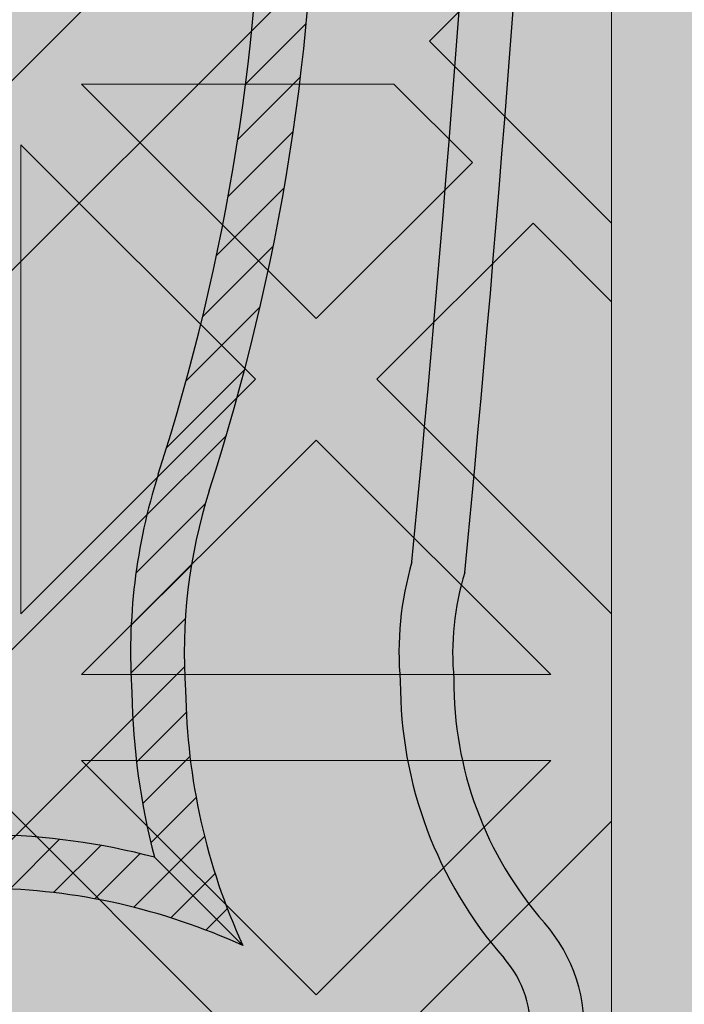
# Model space of a CAD drawing. Units: inches. Extents: x 844 to 2234, y 346 to 1084.
# Tile 10 of 93: x 1125.562 to 1127.536, y 688.258 to 691.183. Entities that reach past the tile are written whole.
import ezdxf

# ---------------------------------------------------------------- set-up
doc = ezdxf.new("R2010")
doc.units = ezdxf.units.IN
doc.header["$MEASUREMENT"] = 0
for name, color, linetype, lineweight in [('A-ANNO-DIMS', 2, 'Continuous', 18), ('furniture', 8, 'Continuous', 18), ('RA-AP-01$0$INT', 35, 'Continuous', 5)]:
    doc.layers.add(name, color=color, linetype=linetype, lineweight=lineweight)
doc.layers.add('RA-AP-01$0$FURN', color=3, linetype='Continuous')
doc.layers.add('RA-AP-01$0$WOOD', color=64, linetype='Continuous')
doc.styles.get("Standard").update_dxf_attribs({"font": 'arial.ttf'})
doc.dimstyles.get("Standard").update_dxf_attribs({"dimtxt": 6, "dimasz": 3, "dimexe": 0.18, "dimexo": 0.0625, "dimgap": 0.09, "dimtad": 0, "dimtih": 1, "dimtoh": 1, "dimdec": 1, "dimzin": 0, "dimdsep": 46, "dimlunit": 3, "dimtxsty": 'Standard', "dimblk": 'ARCHTICK', "dimcen": 0.09, "dimadec": 0, "dimazin": 0, "dimtfac": 1, "dimtdec": 1, "dimtofl": 0, "dimtmove": 0, "dimatfit": 3, "dimfxl": 1, "dimtolj": 1, "dimtzin": 0, "dimarcsym": 0})

# ---------------------------------------------------------------- blocks, each defined once
blk = doc.blocks.new('A$C18D01794')
at = {"layer": 'RA-AP-01$0$INT'}
blk.add_hatch(color=256, dxfattribs=at).paths.add_polyline_path([(4.505206456958071, -6.306712009588038), (5.305206456958072, -6.306712009588038), (5.305206456958072, -7.106712009588038), (5.255206456951893, -7.10671200958804), (5.25520645694868, -6.356712009605972), (4.555206456959269, -6.356712009587461), (4.555206456956052, -7.106712009588038), (4.505206456958073, -7.106712009588038)])
h = blk.add_hatch(color=256, dxfattribs=at)
h.paths.add_polyline_path([(4.585917135068449, -6.356712009588271), (4.555206456959269, -6.35671200958746), (4.555206456959137, -6.387422687716308), (4.874495778835233, -6.706712009592356), (4.90520645695423, -6.676001331474049)])
h.paths.add_polyline_path([(5.255206456948813, -6.387422687716306), (5.255206456948682, -6.356712009605972), (5.224495778822613, -6.356712009605161), (4.905206456953498, -6.676001331474273), (4.935917135072151, -6.706712009592924)])
h.paths.add_polyline_path([(4.935917135072559, -6.706712009592068), (4.905206456953564, -6.737422687710376), (5.255206456951813, -7.087422687708613), (5.255206456951549, -7.026001331471008)])
h.paths.add_polyline_path([(4.555206456956399, -7.026001331471013), (4.555206456956134, -7.087422687708616), (4.905206456953821, -6.737422687710943), (4.874495778835166, -6.70671200959229)])
h = blk.add_hatch(color=256, dxfattribs=at)
h.paths.add_polyline_path([(4.585917135068448, -6.356712009588273), (4.614201406330596, -6.356712009589021), (4.668846067270487, -6.411356670531338), (4.723490728212344, -6.356712009591912), (4.771774999457151, -6.35671200959319), (4.826419660396886, -6.411356670535356), (4.862780050090322, -6.374996280843536), (4.844495778842715, -6.356712009595112), (4.862780050090411, -6.356712009595595), (4.905206456960182, -6.399138416468211), (4.947632863832445, -6.356712009597838), (4.965917135079675, -6.356712009598322), (4.947632863831759, -6.374996280845421), (4.983993253523576, -6.411356670538857), (5.038637914464627, -6.356712009600247), (5.08692218571208, -6.356712009601523), (5.141566846649976, -6.411356670541852), (5.196211507589851, -6.356712009604411), (5.224495778822615, -6.356712009605161), (4.905206456953975, -6.676001331473793)])
h.paths.add_polyline_path([(4.895206456956031, -6.637717060225675), (4.895206456958921, -6.528427738347902), (4.840561796018589, -6.583072399285802)], flags=16)
h.paths.add_polyline_path([(4.915206456955638, -6.637717060226121), (4.969851117895509, -6.583072399288678), (4.915206456957609, -6.528427738348344)], flags=16)
h.paths.add_polyline_path([(4.826419660395175, -6.568930263661755), (4.881064321335613, -6.514285602723745), (4.771774999456703, -6.514285602720857)], flags=16)
h.paths.add_polyline_path([(4.983993253519558, -6.568930263665262), (5.038637914460456, -6.514285602726792), (4.929348592581548, -6.514285602724816)], flags=16)
h.paths.add_polyline_path([(4.881064321336025, -6.494285602723742), (4.826419660397532, -6.439640941782821), (4.771774999457062, -6.494285602720859)], flags=16)
h.paths.add_polyline_path([(4.929348592582019, -6.494285602724817), (5.038637914460982, -6.494285602726792), (4.983993253522945, -6.439640941786327)], flags=16)
h.paths.add_polyline_path([(4.895206456960191, -6.480143467100443), (4.895206456962115, -6.407422687715913), (4.876922185715016, -6.389138416467584), (4.840561796021581, -6.425498806159401)], flags=16)
h.paths.add_polyline_path([(4.915206456958487, -6.480143467100889), (4.969851117899527, -6.425498806162279), (4.933490728206909, -6.389138416468043), (4.9152064569598, -6.40742268771434)], flags=16)
h.paths.add_polyline_path([(4.757632863832376, -6.480143467096812), (4.812277524772842, -6.425498806158772), (4.757632863834348, -6.370854145217844)], flags=16)
h.paths.add_polyline_path([(4.737632863832376, -6.480143467096286), (4.737632863834348, -6.370854145217375), (4.682988202893906, -6.425498806155385)], flags=16)
h.paths.add_polyline_path([(5.05278005008503, -6.480143467103376), (5.052780050087917, -6.370854145224413), (4.998135389146995, -6.425498806162908)], flags=16)
h.paths.add_polyline_path([(5.072780050085024, -6.480143467103744), (5.127424711025931, -6.42549880616527), (5.072780050087916, -6.370854145224832)], flags=16)
h.paths.add_polyline_path([(4.935917135072783, -6.706712009592292), (5.255206456948811, -6.387422687716309), (5.255206456948932, -6.415706958964177), (5.200561796010279, -6.470351619902839), (5.255206456949403, -6.524996280841948), (5.25520645694961, -6.5732805520894), (5.200561796009787, -6.627925213029239), (5.236922185702417, -6.664285602721864), (5.255206456949919, -6.646001331474357), (5.255206456949998, -6.664285602721898), (5.212780050078687, -6.706712009592262), (5.25520645695036, -6.749138416463932), (5.255206456950438, -6.767422687711313), (5.236922185702424, -6.749138416463297), (5.200561796009796, -6.785498806155928), (5.255206456950753, -6.840143467096874), (5.25520645695096, -6.888427738341682), (5.200561796010322, -6.943072399282328), (5.255206456951428, -6.997717060223427), (5.255206456951547, -7.026001331471006)])
h.paths.add_polyline_path([(5.042988202883395, -6.785498806155427), (5.097632863823085, -6.840143467095101), (5.097632863822622, -6.730854145216193)], flags=16)
h.paths.add_polyline_path([(5.028846067259663, -6.771356670531693), (5.083490728198774, -6.716712009592573), (4.974201406321001, -6.716712009593042)], flags=16)
h.paths.add_polyline_path([(5.117632863823087, -6.840143467095186), (5.172277524762331, -6.785498806155926), (5.11763286382262, -6.730854145216225)], flags=16)
h.paths.add_polyline_path([(5.08349072819877, -6.696712009593886), (5.028846067259652, -6.642067348654775), (4.974201406320998, -6.696712009593438)], flags=16)
h.paths.add_polyline_path([(5.131774999446817, -6.854285602718917), (5.186419660386065, -6.799640941779662), (5.241064321325782, -6.854285602719365)], flags=17)
h.paths.add_polyline_path([(5.131774999446228, -6.716712009592374), (5.186419660386065, -6.771356670532194), (5.222780050079488, -6.734996280838764), (5.204495778832781, -6.716712009592063)], flags=16)
h.paths.add_polyline_path([(5.097632863822613, -6.682569873970264), (5.097632863823061, -6.573280552091354), (5.042988202883383, -6.627925213031044)], flags=16)
h.paths.add_polyline_path([(5.131774999446899, -6.874285602718915), (5.241064321325809, -6.874285602719364), (5.186419660386591, -6.928930263658598)], flags=17)
h.paths.add_polyline_path([(5.131774999446226, -6.696712009594078), (5.204495778830767, -6.696712009594374), (5.22278005007868, -6.67842773834687), (5.186419660386049, -6.642067348654249)], flags=16)
h.paths.add_polyline_path([(5.11763286382262, -6.682569873970225), (5.17227752476232, -6.627925213030515), (5.117632863823064, -6.573280552091267)], flags=16)
h.paths.add_polyline_path([(5.186419660386069, -6.613783077405491), (5.241064321325754, -6.559138416465795), (5.131774999446791, -6.559138416466263)], flags=16)
h.paths.add_polyline_path([(5.131774999446872, -6.539138416466263), (5.24106432132578, -6.539138416465794), (5.186419660386554, -6.484493755526573)], flags=16)
h.paths.add_polyline_path([(5.255206456951811, -7.08742268770861), (5.255206456951895, -7.106712009588038), (4.555206456956052, -7.106712009588038), (4.555206456956136, -7.087422687708617), (4.905206456953973, -6.737422687710788)])
h.paths.add_polyline_path([(4.983993253513404, -6.8444937555241), (4.92934859257295, -6.899138416462108), (5.03863791445186, -6.899138416465014)], flags=16)
h.paths.add_polyline_path([(4.969851117889988, -6.83035161990006), (4.915206456952556, -6.775706958960171), (4.915206456949648, -6.884996280837944)], flags=16)
h.paths.add_polyline_path([(4.929348592572535, -6.919138416462105), (4.983993253511019, -6.973783077403037), (5.038637914451496, -6.919138416465012)], flags=16)
h.paths.add_polyline_path([(5.052780050074912, -6.93328055208906), (4.998135389134438, -6.987925213027088), (5.052780050072919, -7.042569873968025)], flags=16)
h.paths.add_polyline_path([(5.07278005007491, -6.933280552089588), (5.072780050072918, -7.042569873968497), (5.127424711013374, -6.987925213030498)], flags=16)
h.paths.add_polyline_path([(4.89520645695295, -6.775706958959721), (4.840561796013067, -6.830351619897157), (4.895206456950961, -6.884996280837494)], flags=16)
h.paths.add_polyline_path([(4.915206456948365, -6.933280552085403), (4.915206456946434, -7.006001331471951), (4.933490728192729, -7.024285602719066), (4.969851117886972, -6.987925213026453)], flags=16)
h.paths.add_polyline_path([(4.881064321327021, -6.899138416461022), (4.82641966038902, -6.84449375552057), (4.771774999448108, -6.899138416459029)], flags=16)
h.paths.add_polyline_path([(4.895206456950073, -6.933280552084951), (4.840561796009022, -6.987925213023558), (4.876922185700835, -7.024285602716997), (4.895206456948749, -7.006001331469487)], flags=16)
h.paths.add_polyline_path([(4.983993253510392, -7.0020673486505), (4.947632863816944, -7.038427738342319), (4.965917135064043, -7.05671200959023), (5.038637914448995, -7.056712009591555)], flags=16)
h.paths.add_polyline_path([(4.881064321326543, -6.91913841646102), (4.771774999447578, -6.919138416459031), (4.826419660385607, -6.973783077399508)], flags=16)
h.paths.add_polyline_path([(4.905206456946447, -7.014285602717636), (4.862780050074785, -7.056712009588352), (4.947632863816685, -7.056712009589775)], flags=16)
h.paths.add_polyline_path([(5.14156684663679, -7.002067348654549), (5.086922185696452, -7.056712009592438), (5.196211507574223, -7.056712009594425)], flags=16)
h.paths.add_polyline_path([(4.8264196603837, -7.002067348646972), (4.771774999442643, -7.056712009585575), (4.8444957788276, -7.056712009587508), (4.862780050075511, -7.038427738340416)], flags=16)
h.paths.add_polyline_path([(4.812277524760289, -6.98792521302292), (4.757632863822258, -6.933280552082447), (4.757632863819352, -7.042569873961408)], flags=16)
h.paths.add_polyline_path([(4.73763286382226, -6.933280552082079), (4.682988202881349, -6.987925213020536), (4.737632863819352, -7.04256987396099)], flags=16)
h.paths.add_polyline_path([(4.723490728195188, -7.056712009584289), (4.668846067257299, -7.002067348643949), (4.614201406317417, -7.056712009581383)], flags=16)
h.paths.add_polyline_path([(4.597632863829262, -6.706712009592262), (4.555206456957951, -6.664285602721896), (4.555206456958029, -6.646001331474357), (4.573490728205535, -6.664285602721864), (4.609851117898167, -6.627925213029238), (4.555206456958338, -6.573280552089402), (4.555206456958546, -6.524996280841952), (4.60985111789767, -6.470351619902839), (4.555206456959015, -6.415706958964177), (4.555206456959138, -6.387422687716309), (4.874495778835167, -6.70671200959229), (4.5552064569564, -7.026001331471015), (4.555206456956523, -6.997717060223433), (4.609851117897629, -6.94307239928233), (4.555206456956988, -6.888427738341681), (4.555206456957198, -6.840143467096881), (4.609851117898153, -6.78549880615593), (4.573490728205528, -6.749138416463297), (4.555206456957507, -6.76742268771132), (4.555206456957585, -6.749138416463933)])
h.paths.add_polyline_path([(4.712780050085332, -6.730854145216195), (4.712780050084863, -6.840143467095105), (4.767424711024555, -6.785498806155427)], flags=16)
h.paths.add_polyline_path([(4.726922185709173, -6.716712009592573), (4.781566846648288, -6.771356670531693), (4.836211507586949, -6.716712009593043)], flags=16)
h.paths.add_polyline_path([(4.692780050085327, -6.730854145216225), (4.638135389145619, -6.785498806155928), (4.692780050084865, -6.840143467095185)], flags=16)
h.paths.add_polyline_path([(4.726922185709182, -6.696712009593886), (4.836211507586949, -6.696712009593436), (4.7815668466483, -6.642067348654773)], flags=16)
h.paths.add_polyline_path([(4.678637914461726, -6.71671200959237), (4.605917135075169, -6.716712009592063), (4.587632863828464, -6.734996280838766), (4.623993253521887, -6.771356670532195)], flags=16)
h.paths.add_polyline_path([(4.712780050085336, -6.68256987397026), (4.767424711024568, -6.627925213031042), (4.71278005008489, -6.573280552091352)], flags=16)
h.paths.add_polyline_path([(4.678637914461726, -6.696712009594076), (4.623993253521899, -6.642067348654247), (4.587632863829271, -6.67842773834687), (4.605917135077185, -6.696712009594376)], flags=16)
h.paths.add_polyline_path([(4.692780050085336, -6.682569873970228), (4.692780050084889, -6.573280552091267), (4.638135389145632, -6.627925213030515)], flags=16)
h.paths.add_polyline_path([(4.623993253521885, -6.799640941779662), (4.678637914461131, -6.854285602718915), (4.56934859258217, -6.854285602719365)], flags=17)
h.paths.add_polyline_path([(4.623993253521901, -6.613783077405509), (4.678637914461158, -6.559138416466263), (4.569348592582195, -6.559138416465795)], flags=16)
h.paths.add_polyline_path([(4.678637914461051, -6.874285602718915), (4.623993253521361, -6.928930263658598), (4.569348592582143, -6.874285602719364)], flags=17)
h.paths.add_polyline_path([(4.678637914461076, -6.539138416466263), (4.623993253521399, -6.484493755526573), (4.569348592582167, -6.539138416465796)], flags=16)
h = blk.add_hatch(color=256, dxfattribs=at)
h.paths.add_polyline_path([(5.028846067259997, -6.642067348655121), (4.974201406321342, -6.696712009593783), (5.083490728199115, -6.69671200959423)])
h.paths.add_polyline_path([(4.974201406321344, -6.716712009593388), (5.028846067260004, -6.771356670532039), (5.083490728199117, -6.716712009592919)])
h.paths.add_polyline_path([(5.042988202883738, -6.785498806155768), (5.097632863823428, -6.840143467095449), (5.097632863822963, -6.73085414521654)])
h.paths.add_polyline_path([(5.117632863822961, -6.730854145216568), (5.117632863823428, -6.840143467095531), (5.172277524762674, -6.785498806156272)])
h.paths.add_polyline_path([(5.131774999446572, -6.716712009592718), (5.186419660386406, -6.77135667053254), (5.222780050079831, -6.734996280839116), (5.204495778833122, -6.716712009592409)])
h.paths.add_polyline_path([(5.236922185702764, -6.749138416463644), (5.200561796010139, -6.785498806156274), (5.255206456949971, -6.840143467096101), (5.255206456950271, -6.76742268771115)])
h.paths.add_polyline_path([(5.186419660386412, -6.799640941780006), (5.131774999447164, -6.854285602719262), (5.241064321326123, -6.854285602719711)])
h.paths.add_polyline_path([(5.131774999447238, -6.874285602719261), (5.186419660386934, -6.928930263658944), (5.241064321326153, -6.874285602719709)])
h.paths.add_polyline_path([(5.200561796010663, -6.943072399282675), (5.255206456949324, -6.997717060221329), (5.255206456949777, -6.888427738343558)])
h.paths.add_polyline_path([(5.21278005007903, -6.706712009592607), (5.255206456950223, -6.749138416463798), (5.255206456950696, -6.664285602721891)])
h.paths.add_polyline_path([(5.13177499944657, -6.696712009594424), (5.204495778831106, -6.696712009594723), (5.222780050079024, -6.678427738347219), (5.186419660386397, -6.642067348654592)])
h.paths.add_polyline_path([(5.117632863823405, -6.573280552091611), (5.117632863822955, -6.682569873970578), (5.172277524762665, -6.627925213030859)])
h.paths.add_polyline_path([(5.042988202883727, -6.627925213031387), (5.097632863822957, -6.682569873970603), (5.097632863823407, -6.573280552091697)])
h.paths.add_polyline_path([(5.131774999447135, -6.559138416466609), (5.186419660386394, -6.613783077405857), (5.241064321326097, -6.559138416466144)])
h.paths.add_polyline_path([(5.200561796010128, -6.627925213029584), (5.236922185702758, -6.664285602722211), (5.255206456950264, -6.646001331474705), (5.255206456949948, -6.573280552089752)])
h.paths.add_polyline_path([(5.186419660386895, -6.484493755526919), (5.131774999447213, -6.539138416466609), (5.241064321326127, -6.539138416466142)])
h.paths.add_polyline_path([(5.200561796010624, -6.470351619903183), (5.255206456949745, -6.524996280842298), (5.255206456949276, -6.415706958964523)])
for p, q in [((5.255206456951895, -7.106712009588038), (5.255206456948681, -6.356712009605972)), ((4.935917135072783, -6.706712009592292), (5.255206456948813, -6.387422687716307)), ((5.255206456949399, -6.524996280841946), (5.200561796010281, -6.470351619902839)), ((5.18641966038655, -6.484493755526575), (5.131774999446872, -6.539138416466263)), ((5.241064321325782, -6.539138416465796), (5.186419660386552, -6.484493755526573)), ((5.131774999446872, -6.539138416466263), (5.241064321325782, -6.539138416465796)), ((5.131774999446792, -6.559138416466263), (5.241064321325755, -6.559138416465795)), ((5.131774999446792, -6.559138416466263), (5.186419660386049, -6.613783077405509)), ((5.241064321325755, -6.559138416465795), (5.186419660386049, -6.613783077405509)), ((5.117632863823062, -6.573280552091267), (5.172277524762319, -6.627925213030515)), ((5.117632863823062, -6.573280552091267), (5.117632863822614, -6.68256987397023)), ((5.255206456949605, -6.573280552089405), (5.200561796009783, -6.627925213029239)), ((5.255206456949918, -6.646001331474357), (5.255206456949605, -6.573280552089405)), ((5.117632863822614, -6.68256987397023), (5.172277524762319, -6.627925213030515)), ((5.200561796009783, -6.627925213029238), (5.236922185702415, -6.664285602721863)), ((5.131774999446228, -6.696712009594078), (5.186419660386053, -6.642067348654247)), ((5.186419660386051, -6.642067348654247), (5.222780050078681, -6.67842773834687)), ((5.255206456949919, -6.646001331474357), (5.236922185702415, -6.664285602721864)), ((5.212780050078687, -6.706712009592262), (5.255206456950353, -6.664285602721543)), ((5.25520645694988, -6.74913841646345), (5.255206456950353, -6.664285602721543)), ((5.204495778833082, -6.69671200959206), (5.222780050078681, -6.67842773834687)), ((5.204495778831179, -6.696712009594376), (5.131774999446228, -6.696712009594078)), ((5.212780050078687, -6.706712009592262), (5.25520645694988, -6.74913841646345))]:
    blk.add_line(p, q, dxfattribs=at)
blk = doc.blocks.new('A$C32926AE1')
at = {"layer": 'RA-AP-01$0$WOOD'}
h = blk.add_hatch(color=256, dxfattribs=at)
h.dxf.hatch_style = 1
h.paths.add_polyline_path([(5.157430609644524, 4.573483066760929, -0.1009492694046607), (5.155401577623758, 4.593365984175333, -0.1842662638101597), (5.172249623284174, 4.638795604568598, 0.2056608120311276), (5.179560981299304, 4.661316324430096, 0.3614336704623542), (5.134352340494423, 4.706524965234944, 0.2056608120311297), (5.111831620632933, 4.699213607219793, -0.1842662638101113), (5.066402000239693, 4.682365561559342, -0.1055311479399994), (5.045656153913092, 4.68467289944697, 0.1567636581983829), (4.763886414745334, 4.684672899446966, -0.1055311479399895), (4.743140568418733, 4.68236556155934, -0.1842662638100833), (4.6977109480255, 4.69921360721979, 0.2056608120302612), (4.675190228164109, 4.706524965234949, 0.3614336704708441), (4.629981587358889, 4.66131632442871, 0.2056608120245944), (4.637292945374126, 4.638795604567974, -0.1842662638101024), (4.654140991034615, 4.59336598417475, -0.1009492694055169), (4.652111959013835, 4.573483066760181, 0.021410119221476), (4.629748025606143, 4.156712009541676, 0.0214101192214795), (4.652111959013809, 3.739940952323101, -0.1009492694059586), (4.654140991034615, 3.720058034908448, -0.1842662638100975), (4.637292945374126, 3.674628414515226, 0.2056608120245705), (4.629981587358889, 3.652107694654492, 0.3614336704708879), (4.675190228164113, 3.606899053848249, 0.2056608120302384), (4.697710948025501, 3.614210411863408, -0.1842662638100995), (4.743140568418738, 3.63105845752386, -0.1055311479402541), (4.763886414745388, 3.628751119636215, 0.1567636581983776), (5.045656153913137, 3.628751119636244, -0.1055311479397538), (5.066402000239692, 3.631058457523857, -0.1842662638101067), (5.111831620632931, 3.614210411863407, 0.2056608120310924), (5.134352340494417, 3.606899053848256, 0.3614336704624001), (5.179560981299307, 3.652107694653103, 0.2056608120311314), (5.172249623284175, 3.6746284145146, -0.1842662638101402), (5.155401577623758, 3.72005803490786, -0.1009492694051366), (5.15743060964455, 3.739940952322354, 0.0214101192215073), (5.179794543052287, 4.156712009541468, 0.0214101192215252)])
h.paths.add_polyline_path([(4.639748609479751, 4.156712009541513, 0.0213537860821624), (4.661970494867118, 3.741887061152232, -0.094075836301374), (4.664143710413708, 3.7196126951003, -0.1824818158568985), (4.644813765429836, 3.668037719127816, 0.2056608120245319), (4.639939526753007, 3.653023905887301, 0.3614336704710246), (4.676106439397173, 3.616856993242342, 0.2056608120302234), (4.691120252638095, 3.621731231919122, -0.1824818158602558), (4.742695228611606, 3.641061176902986, -0.1029891339458722), (4.766991894714349, 3.638256818950944, 0.156709409989566), (5.042550673941472, 3.638256818950105, -0.102989133958497), (5.066847340047078, 3.641061176902949, -0.1824818158594995), (5.118422316020358, 3.621731231919103, 0.2056608120311416), (5.133436129261316, 3.616856993242346, 0.3614336704621468), (5.169603041905217, 3.653023905886178, 0.2056608120310986), (5.164728803228477, 3.668037719127177, -0.1824818158565612), (5.145398858244737, 3.719612695099578, -0.0940758363009313), (5.147572073791232, 3.741887061151398, 0.0213537860822023), (5.169793959178681, 4.156712009541451, 0.0213537860822226), (5.147572073791203, 4.571536957931898, -0.0940758363005034), (5.145398858244737, 4.59381132398362, -0.1824818158565587), (5.164728803228476, 4.645386299956021, 0.2056608120311045), (5.169603041905216, 4.66040011319702, 0.3614336704621845), (5.133436129261313, 4.696567025840856, 0.2056608120310773), (5.118422316020359, 4.691692787164098, -0.182481815859508), (5.066847340047078, 4.67236284218025, -0.1029891339584606), (5.04255067394148, 4.675167200133092, 0.156709409989566), (4.766991894714357, 4.675167200132257, -0.1029891339458842), (4.742695228611611, 4.672362842180213, -0.1824818158602725), (4.691120252638095, 4.691692787164077, 0.2056608120302152), (4.676106439397174, 4.696567025840858, 0.3614336704710363), (4.639939526753005, 4.660400113195899, 0.2056608120245495), (4.644813765429837, 4.645386299955384, -0.1824818158568934), (4.664143710413708, 4.593811323982902, -0.0940758363009187), (4.661970494867149, 4.571536957931074, 0.021353786082177)], flags=16)
h.paths.add_polyline_path([(5.129794543052235, 4.432167055276933, -0.0141661062790638), (5.130152669293814, 4.156927903047693, -0.0141661062790647), (5.129794543052234, 3.881688750818433, -0.0785247771143638), (5.10979738006795, 3.755143611847103, 0.0945969212073497), (5.105408519571111, 3.717898134952927, 0.1043170707844957), (5.116074640131521, 3.670385395016088, 0.1043170707864965), (5.068561900193738, 3.681051515576561, 0.09459692119553), (5.031316423304057, 3.676662655080835, -0.1580239521427272), (4.778226145355827, 3.676662655080367, 0.0945969211986668), (4.740980668464973, 3.681051515576592, 0.1043170707882822), (4.693467928526415, 3.670385395015844, 0.1043170707867916), (4.704134049087309, 3.717898134953662, 0.0945969211972894), (4.69974518859162, 3.755143611844042, -0.0785247771163196), (4.679748025606343, 3.881688750818406, -0.0141661062790663), (4.679389899364763, 4.156927903047693, -0.0141661062790672), (4.679748025606343, 4.432167055276998, -0.0785247771163064), (4.699745188591625, 4.55871219425134, 0.094596921197333), (4.704134049087308, 4.595957671141738, 0.1043170707867205), (4.693467928526416, 4.643470411079523, 0.1043170707882628), (4.740980668464965, 4.632804290518776, 0.0945969211988114), (4.778226145355874, 4.637193151015016, -0.158023952142669), (5.031316423304015, 4.637193151014546, 0.0945969211956361), (5.068561900193736, 4.632804290518806, 0.1043170707864979), (5.11607464013152, 4.643470411079278, 0.1043170707844617), (5.105408519571112, 4.595957671142455, 0.0945969212074597), (5.109797380067959, 4.558712194248236, -0.0785247771143467)], flags=0)
h.paths.add_polyline_path([(5.119794532311105, 4.432259799204851, -0.0142000800617244), (5.120156169157484, 4.156927903047701, -0.0142000800617277), (5.119794532311105, 3.881596006890482, -0.0784894509520253), (5.100273383573699, 3.758192358677797, 0.0940138827242913), (5.095413455884425, 3.717477693979438, 0.0606271852308753), (5.099615656341024, 3.686844378806616, 0.0606271852322524), (5.068982341167493, 3.691046579263239, 0.0940138827010453), (5.028267676478798, 3.686186651576848, -0.1580706864508061), (4.781274892180912, 3.686186651576435, 0.0940138827026903), (4.740560227491556, 3.691046579263279, 0.0606271852339895), (4.709926912317155, 3.686844378806508, 0.0606271852329405), (4.714129112773991, 3.717477693980356, 0.094013882701304), (4.709269185087677, 3.758192358669163, -0.0784894509577193), (4.689748036347473, 3.881596006890469, -0.014200080061729), (4.689386399501094, 4.156927903047709, -0.0142000800617217), (4.689748036347473, 4.432259799204808, -0.078489450957724), (4.709269185087651, 4.555663447426125, 0.0940138827014585), (4.714129112773992, 4.596378112114996, 0.0606271852329731), (4.709926912317154, 4.62701142728886, 0.0606271852340196), (4.74056022749157, 4.622809226832087, 0.0940138827024997), (4.781274892180847, 4.627669154518912, -0.1580706864508359), (5.028267676478777, 4.627669154518526, 0.0940138827010946), (5.068982341167492, 4.622809226832129, 0.060627185232254), (5.099615656341024, 4.627011427288751, 0.0606271852308727), (5.095413455884425, 4.59637811211593, 0.0940138827241088), (5.100273383573675, 4.555663447417647, -0.0784894509520978)], flags=0)
h.paths.add_polyline_path([(5.06978912287499, 4.430218106756144, -0.014241683694547), (5.070173729147532, 4.156927903047672, -0.0142416836945458), (5.06978912287499, 3.883637699339223, -0.0800609523125196), (5.052662118612511, 3.773463122773442, 0.0526421978001116), (5.04590916754064, 3.740550867606997, 0.0526421977992423), (5.012996912374707, 3.73379791653534, -0.1583028414718258), (4.796545656286308, 3.73379791653451, 0.0526421978034211), (4.763633401117837, 3.740550867607021, 0.0526421978018622), (4.756880450045755, 3.773463122774558, -0.0800609523117106), (4.739753445783639, 3.883637699339268, -0.0142416836945435), (4.739368839511098, 4.156927903047671, -0.0142416836945477), (4.739753445783639, 4.430218106756155, -0.0800609523116345), (4.75688045004574, 4.540392683320762, 0.052642197801941), (4.763633401117837, 4.573304938488346, 0.0526421978035071), (4.796545656286361, 4.580057889560873, -0.1583028414717561), (5.012996912374669, 4.580057889560039, 0.0526421977993048), (5.04590916754064, 4.57330493848837, 0.0526421978002057), (5.052662118612529, 4.540392683321868, -0.080060952312477)], flags=0)
h.paths.add_polyline_path([(5.049789715110557, 4.43038092723357, -0.0143097550741839), (5.05018085590259, 4.156927903047715, -0.0143097550741854), (5.049789715110558, 3.883474878861827, -0.0800685599149176), (5.03362098255317, 3.779581877367999, 0.0306258898956367), (5.028241146483733, 3.758218888663947, 0.0306258898977031), (5.006878157778253, 3.75283905259408, -0.1583983521624096), (4.802664410878162, 3.752839052594731, 0.0306258898946014), (4.781301422174808, 3.758218888663924, 0.0306258898967912), (4.775921586105202, 3.779581877368794, -0.080068559914251), (4.759752853548071, 3.883474878861786, -0.0143097550741854), (4.759361712756037, 4.156927903047671, -0.0143097550741854), (4.759752853548071, 4.430380927233557, -0.0800685599142479), (4.775921586105193, 4.534273928726546, 0.0306258898968306), (4.781301422174808, 4.555636917431444, 0.0306258898945754), (4.802664410878143, 4.561016753500631, -0.1583983521624168), (5.006878157778244, 4.561016753501291, 0.0306258898977177), (5.028241146483733, 4.555636917431421, 0.0306258898958182), (5.03362098255321, 4.534273928727244, -0.080068559914796)], flags=0)
h.paths.add_polyline_path([(4.999766070382627, 4.428171244713864, -0.0143443147609634), (5.000198441819402, 4.156927903047689, -0.0143443147609612), (4.999766070382627, 3.885684561381556, -0.0784641635803329), (4.987356730658798, 3.799103304488872, -0.1506053783831347), (4.822185837999821, 3.79910330448882, -0.0784641635803318), (4.809776498276007, 3.885684561381509, -0.014344314760963), (4.809344126839227, 4.156927903047677, -0.0143443147609645), (4.809776498276007, 4.428171244713873, -0.0784641635803192), (4.822185837999822, 4.514752501606549, -0.1506053783831338), (4.987356730658798, 4.514752501606494, -0.078464163580285)], flags=0)
h.paths.add_polyline_path([(4.979755254238824, 4.42764379880488, -0.0143772539198268), (4.980205517789977, 4.156927903047693, -0.0143772539198275), (4.979755254238824, 3.886212007290489, -0.0689242507424422), (4.971183264704897, 3.815276770442801, -0.1296645318904179), (4.838359303953726, 3.815276770442746, -0.0689242507424186), (4.829787314419809, 3.886212007290419, -0.0143772539198292), (4.829337050868653, 4.156927903047653, -0.0143772539198325), (4.829787314419809, 4.427643798804946, -0.0689242507424211), (4.838359303953725, 4.498579035652621, -0.1296645318904187), (4.971183264704897, 4.498579035652565, -0.0689242507424401)], flags=0)
h = blk.add_hatch(color=256, dxfattribs=at)
h.dxf.hatch_style = 1
h.paths.add_polyline_path([(5.145398858244737, 4.59381132398362, -0.1824818158565616), (5.164728803228476, 4.645386299956021, 0.2056608120311045), (5.169603041905216, 4.66040011319702, 0.3614336704621845), (5.133436129261313, 4.696567025840856, 0.2056608120310773), (5.118422316020359, 4.691692787164098, -0.182481815859508), (5.066847340047078, 4.67236284218025, -0.1029891339584606), (5.04255067394148, 4.675167200133092, 0.156709409989566), (4.766991894714357, 4.675167200132257, -0.1029891339458842), (4.742695228611611, 4.672362842180213, -0.1824818158602725), (4.691120252638095, 4.691692787164077, 0.2056608120302152), (4.676106439397174, 4.696567025840858, 0.3614336704710363), (4.639939526753005, 4.660400113195899, 0.2056608120245495), (4.644813765429837, 4.645386299955384, -0.1824818158568934), (4.664143710413708, 4.593811323982902, -0.0940758363009187), (4.661970494867149, 4.571536957931074, 0.0213537860821772), (4.639748609479751, 4.156712009541507, 0.0213537860821625), (4.661970494867119, 3.741887061152226, -0.0940758363013071), (4.664143710413708, 3.719612695100309, -0.1824818158569294), (4.644813765429836, 3.668037719127816, 0.2056608120245319), (4.639939526753007, 3.653023905887301, 0.3614336704710246), (4.676106439397173, 3.616856993242342, 0.2056608120302234), (4.691120252638095, 3.621731231919122, -0.1824818158602558), (4.742695228611606, 3.641061176902986, -0.1029891339458722), (4.766991894714349, 3.638256818950944, 0.156709409989566), (5.042550673941472, 3.638256818950105, -0.102989133958497), (5.066847340047078, 3.641061176902949, -0.1824818158594995), (5.118422316020358, 3.621731231919103, 0.2056608120311416), (5.133436129261316, 3.616856993242346, 0.3614336704621468), (5.169603041905217, 3.653023905886178, 0.2056608120310986), (5.164728803228477, 3.668037719127177, -0.1824818158565612), (5.145398858244737, 3.719612695099578, -0.0940758363009313), (5.147572073791232, 3.741887061151398, 0.0213537860822023), (5.169793959178681, 4.156712009541451, 0.0213537860822226), (5.147572073791203, 4.571536957931898, -0.0940758363004996)])
h.paths.add_polyline_path([(5.109797380067958, 4.55871219424824, -0.0785247771143472), (5.129794543052234, 4.432167055276936, -0.0141661062790644), (5.130152669293814, 4.156927903047685, -0.014166106279066), (5.129794543052234, 3.881688750818401, -0.0785247771143517), (5.109797380067946, 3.755143611847092, 0.0945969212073132), (5.105408519571111, 3.717898134952929, 0.1043170707844995), (5.116074640131521, 3.670385395016088, 0.1043170707864965), (5.068561900193738, 3.681051515576561, 0.09459692119553), (5.031316423304057, 3.676662655080835, -0.1580239521427272), (4.778226145355827, 3.676662655080367, 0.0945969211986668), (4.740980668464973, 3.681051515576592, 0.1043170707882822), (4.693467928526415, 3.670385395015844, 0.1043170707867916), (4.704134049087309, 3.717898134953662, 0.0945969211972894), (4.69974518859162, 3.755143611844042, -0.0785247771163196), (4.679748025606343, 3.881688750818406, -0.0141661062790663), (4.679389899364763, 4.156927903047693, -0.0141661062790672), (4.679748025606343, 4.432167055276998, -0.0785247771163064), (4.699745188591625, 4.55871219425134, 0.094596921197333), (4.704134049087308, 4.595957671141738, 0.1043170707867205), (4.693467928526416, 4.643470411079523, 0.1043170707882628), (4.740980668464965, 4.632804290518776, 0.0945969211988114), (4.778226145355874, 4.637193151015016, -0.158023952142669), (5.031316423304015, 4.637193151014546, 0.0945969211956361), (5.068561900193736, 4.632804290518806, 0.1043170707864979), (5.11607464013152, 4.643470411079278, 0.1043170707844617), (5.105408519571112, 4.595957671142455, 0.0945969212074504)], flags=16)
h.paths.add_polyline_path([(5.100273383573655, 4.55566344741771, -0.0784894509521388), (5.119794532311105, 4.432259799204852, -0.0142000800617252), (5.120156169157484, 4.156927903047686, -0.014200080061726), (5.119794532311105, 3.881596006890502, -0.0784894509520446), (5.100273383573696, 3.758192358677786, 0.0940138827242721), (5.095413455884425, 3.717477693979436, 0.0606271852308692), (5.099615656341024, 3.686844378806616, 0.0606271852322522), (5.068982341167493, 3.691046579263239, 0.0940138827010453), (5.028267676478798, 3.686186651576848, -0.1580706864508061), (4.781274892180912, 3.686186651576435, 0.0940138827026903), (4.740560227491556, 3.691046579263279, 0.0606271852339895), (4.709926912317155, 3.686844378806508, 0.0606271852329405), (4.714129112773991, 3.717477693980356, 0.094013882701304), (4.709269185087677, 3.758192358669163, -0.0784894509577193), (4.689748036347473, 3.881596006890469, -0.014200080061729), (4.689386399501094, 4.156927903047709, -0.0142000800617217), (4.689748036347473, 4.432259799204808, -0.078489450957724), (4.709269185087651, 4.555663447426125, 0.0940138827014585), (4.714129112773992, 4.596378112114996, 0.0606271852329731), (4.709926912317154, 4.62701142728886, 0.0606271852340196), (4.74056022749157, 4.622809226832087, 0.0940138827024997), (4.781274892180847, 4.627669154518912, -0.1580706864508359), (5.028267676478777, 4.627669154518526, 0.0940138827010946), (5.068982341167492, 4.622809226832129, 0.060627185232254), (5.099615656341024, 4.627011427288751, 0.0606271852308727), (5.095413455884425, 4.59637811211593, 0.094013882723957)], flags=0)
h.paths.add_polyline_path([(5.04590916754064, 4.57330493848837, 0.0526421978002057), (5.052662118612529, 4.540392683321868, -0.0800609523124783), (5.06978912287499, 4.430218106756142, -0.0142416836945469), (5.070173729147532, 4.156927903047672, -0.0142416836945458), (5.06978912287499, 3.883637699339223, -0.0800609523125196), (5.052662118612511, 3.773463122773442, 0.0526421978001116), (5.04590916754064, 3.740550867606997, 0.0526421977992423), (5.012996912374707, 3.73379791653534, -0.1583028414718258), (4.796545656286308, 3.73379791653451, 0.0526421978034211), (4.763633401117837, 3.740550867607021, 0.0526421978018622), (4.756880450045755, 3.773463122774558, -0.0800609523117106), (4.739753445783639, 3.883637699339268, -0.0142416836945435), (4.739368839511098, 4.156927903047671, -0.0142416836945477), (4.739753445783639, 4.430218106756155, -0.0800609523116345), (4.75688045004574, 4.540392683320762, 0.052642197801941), (4.763633401117837, 4.573304938488346, 0.0526421978035071), (4.796545656286361, 4.580057889560873, -0.1583028414717561), (5.012996912374669, 4.580057889560039, 0.0526421977993048)], flags=0)
h.paths.add_polyline_path([(5.028241146483733, 4.555636917431422, 0.0306258898956949), (5.033620982553182, 4.534273928727329, -0.0800685599148649), (5.049789715110557, 4.430380927233569, -0.0143097550741839), (5.05018085590259, 4.156927903047715, -0.0143097550741854), (5.049789715110558, 3.883474878861827, -0.0800685599149176), (5.03362098255317, 3.779581877367999, 0.0306258898956367), (5.028241146483733, 3.758218888663947, 0.0306258898977031), (5.006878157778253, 3.75283905259408, -0.1583983521624096), (4.802664410878162, 3.752839052594731, 0.0306258898946014), (4.781301422174808, 3.758218888663924, 0.0306258898967912), (4.775921586105202, 3.779581877368794, -0.080068559914251), (4.759752853548071, 3.883474878861786, -0.0143097550741854), (4.759361712756037, 4.156927903047671, -0.0143097550741854), (4.759752853548071, 4.430380927233557, -0.0800685599142479), (4.775921586105193, 4.534273928726546, 0.0306258898968306), (4.781301422174808, 4.555636917431444, 0.0306258898945754), (4.802664410878143, 4.561016753500631, -0.1583983521624168), (5.006878157778244, 4.561016753501291, 0.0306258898977174)], flags=0)
h.paths.add_polyline_path([(4.987356730658798, 4.514752501606494, -0.0784641635803018), (4.999766070382627, 4.428171244713845, -0.0143443147609637), (5.000198441819402, 4.156927903047665, -0.0143443147609622), (4.999766070382628, 3.885684561381514, -0.0784641635802952), (4.987356730658797, 3.799103304488872, -0.1506053783831338), (4.822185837999821, 3.799103304488819, -0.0784641635803342), (4.809776498276007, 3.885684561381512, -0.0143443147609628), (4.809344126839227, 4.156927903047676, -0.0143443147609646), (4.809776498276007, 4.428171244713873, -0.0784641635803192), (4.822185837999822, 4.514752501606549, -0.1506053783831338)], flags=0)
h.paths.add_polyline_path([(4.971183264704897, 4.498579035652566, -0.0689242507424384), (4.979755254238824, 4.427643798804883, -0.0143772539198276), (4.980205517789977, 4.15692790304768, -0.0143772539198258), (4.979755254238823, 3.88621200729051, -0.0689242507424628), (4.971183264704897, 3.815276770442801, -0.129664531890417), (4.838359303953726, 3.815276770442746, -0.0689242507424186), (4.829787314419809, 3.886212007290419, -0.0143772539198292), (4.829337050868653, 4.156927903047653, -0.0143772539198325), (4.829787314419809, 4.427643798804946, -0.0689242507424211), (4.838359303953725, 4.498579035652621, -0.1296645318904187)], flags=0)
h = blk.add_hatch(dxfattribs=at)
h.set_pattern_fill('ANSI31', color=256, scale=0.05, style=0)
h.set_pattern_definition([(45, (0, 0), (-0.0044194173824159, 0.0044194173824159), [])])
h.paths.add_polyline_path([(5.130152669293814, 4.156927903047704, 0.0141661062790657), (5.129794543052234, 4.432167055276982, 0.0777827904001433), (5.110168979996553, 4.557559993161921, -0.0976515123401879), (5.105408519571111, 4.595957671142454, -0.1043170707844687), (5.116074640131522, 4.64347041107928), (5.099615656341024, 4.627011427288751, 0.0606271852308727), (5.095413455884425, 4.59637811211593, 0.0940138827241088), (5.100273383573675, 4.555663447417647, -0.0784894509520972), (5.119794532311105, 4.432259799204852, -0.0142000800617252), (5.120156169157484, 4.156927903047686, -0.014200080061726), (5.119794532311105, 3.881596006890502, -0.0784894509520446), (5.100273383573696, 3.758192358677786, 0.0940138827242721), (5.095413455884425, 3.717477693979436, 0.0606271852308692), (5.099615656341024, 3.686844378806616), (5.116074640131519, 3.67038539501609, -0.1043170707844594), (5.105408519571112, 3.717898134952912, -0.0976515123401594), (5.11016897999655, 3.756295812933435, 0.0777827904001654), (5.129794543052234, 3.881688750818409, 0.0141661062790665)])
h.paths.add_polyline_path([(5.030164222210597, 3.676291055149937, -0.0976515123472002), (5.068561900193739, 3.681051515576561, -0.1043170707864927), (5.116074640131521, 3.670385395016088), (5.099615656341024, 3.686844378806616, 0.0606271852322522), (5.068982341167493, 3.691046579263239, 0.0940138827010453), (5.028267676478798, 3.686186651576848, -0.1580706864508061), (4.781274892180912, 3.686186651576435, 0.0940138827026903), (4.740560227491556, 3.691046579263279, 0.0606271852339913), (4.709926912317154, 3.686844378806508), (4.693467928526416, 3.670385395015845, -0.1043170707882796), (4.740980668464973, 3.681051515576592, -0.0976515123427246), (4.779378346446416, 3.676291055150394, 0.156512506893803)])
h.paths.add_polyline_path([(4.689748036347473, 3.881596006890472, -0.014200080061729), (4.689386399501094, 4.156927903047712, -0.0142000800617195), (4.689748036347473, 4.432259799204768, -0.078489450957742), (4.709269185087648, 4.555663447426114, 0.0940138827014821), (4.714129112773992, 4.596378112114995, 0.0606271852329748), (4.709926912317154, 4.62701142728886), (4.693467928526414, 4.643470411079524, -0.1043170707867939), (4.704134049087309, 4.595957671141706, -0.09765151234893), (4.699373588660725, 4.557559993157876, 0.0777827903975372), (4.679748025606343, 4.432167055276987, 0.0141661062790675), (4.679389899364763, 4.156927903047675, 0.0141661062790641), (4.679748025606343, 3.88168875081843, 0.0777827903975637), (4.699373588660724, 3.756295812937497, -0.0976515123490278), (4.704134049087308, 3.717898134953629, -0.1043170707867196), (4.693467928526416, 3.670385395015845), (4.709926912317155, 3.686844378806508, 0.0606271852329413), (4.714129112773991, 3.717477693980357, 0.0940138827013084), (4.709269185087676, 3.758192358669166, -0.0784894509577192)])
h.paths.add_polyline_path([(4.779378346446434, 4.63756475094498, -0.0976515123427943), (4.740980668464964, 4.632804290518776, -0.1043170707882609), (4.693467928526416, 4.643470411079523), (4.709926912317154, 4.62701142728886, 0.0606271852340196), (4.74056022749157, 4.622809226832087, 0.0940138827024997), (4.781274892180847, 4.627669154518912, -0.1580706864508359), (5.028267676478777, 4.627669154518526, 0.0940138827010946), (5.068982341167492, 4.622809226832129, 0.060627185232254), (5.099615656341024, 4.627011427288751), (5.116074640131521, 4.643470411079279, -0.1043170707865022), (5.068561900193735, 4.632804290518806, -0.0976515123475899), (5.030164222210446, 4.637564750945479, 0.1565125068936924)])
h = blk.add_hatch(dxfattribs=at)
h.set_pattern_fill('ANSI32', color=256, scale=0.2, style=0)
h.set_pattern_definition([(45, (0, 0), (-0.0530330085889911, 0.0530330085889911), []), (45, (0.035355339, 0), (-0.0530330085889911, 0.0530330085889911), [])])
h.paths.add_polyline_path([(5.119794532311105, 4.432259799204823, 0.0777015974868765), (5.10065834347252, 4.554469821747928, -0.0968902511992216), (5.095413455884425, 4.596378112115931, -0.060627185230871), (5.099615656341024, 4.627011427288751, -0.060627185232254), (5.068982341167492, 4.622809226832129, -0.0968902512198245), (5.027074050790956, 4.628054114423209, 0.1564657949319105), (4.782468517866163, 4.628054114422785, -0.0968902512152247), (4.740560227491555, 4.622809226832088, -0.0606271852339878), (4.709926912317155, 4.627011427288859, -0.0606271852329413), (4.714129112773991, 4.596378112115011, -0.0968902512205338), (4.708884225182929, 4.554469821738175, 0.0777015974804443), (4.689748036347473, 4.43225979920482, 0.0142000800617215), (4.689386399501094, 4.156927903047726, 0.0142000800617273), (4.689748036347473, 3.88159600689052, 0.077701597480541), (4.708884225182985, 3.759385984357019, -0.096890251220082), (4.714129112773992, 3.717477693980371, -0.0606271852329731), (4.709926912317154, 3.686844378806507, -0.060627185233988), (4.740560227491554, 3.691046579263279, -0.0968902512152569), (4.782468517866175, 3.685801691672578, 0.1564657949319236), (5.027074050790988, 3.685801691672169, -0.0968902512197451), (5.068982341167491, 3.691046579263239, -0.0606271852322557), (5.099615656341024, 3.686844378806616, -0.0606271852308727), (5.095413455884425, 3.717477693979438, -0.0968902511991229), (5.100658343472507, 3.7593859843474, 0.0777015974868745), (5.119794532311105, 3.8815960068905, 0.014200080061726), (5.120156169157484, 4.156927903047685, 0.0142000800617238)])
h.paths.add_polyline_path([(5.070173729147531, 4.156927903047684, -0.0142416836945481), (5.06978912287499, 3.883637699339191, -0.0800609523125107), (5.052662118612505, 3.773463122773424, 0.0526421978000811), (5.04590916754064, 3.740550867606997, 0.0526421977993214), (5.012996912374658, 3.733797916535325, -0.1583028414717916), (4.796545656286304, 3.733797916534512, 0.0526421978034138), (4.763633401117837, 3.740550867607021, 0.0526421978018622), (4.756880450045755, 3.773463122774558, -0.0800609523117106), (4.739753445783639, 3.883637699339268, -0.0142416836945435), (4.739368839511098, 4.156927903047671, -0.0142416836945477), (4.739753445783639, 4.430218106756155, -0.0800609523116345), (4.75688045004574, 4.540392683320762, 0.052642197801941), (4.763633401117837, 4.573304938488346, 0.0526421978035071), (4.796545656286361, 4.580057889560873, -0.1583028414717561), (5.012996912374669, 4.580057889560039, 0.0526421977993048), (5.04590916754064, 4.57330493848837, 0.0526421978002057), (5.052662118612529, 4.540392683321868, -0.0800609523124783), (5.06978912287499, 4.430218106756142, -0.0142416836945463)], flags=16)
h.paths.add_polyline_path([(5.050180855902591, 4.156927903047686, -0.0143097550741856), (5.049789715110558, 3.883474878861795, -0.0800685599148126), (5.033620982553202, 3.7795818773681, 0.0306258898957837), (5.028241146483733, 3.758218888663947, 0.0306258898977031), (5.006878157778253, 3.75283905259408, -0.1583983521624096), (4.802664410878162, 3.752839052594731, 0.0306258898946014), (4.781301422174808, 3.758218888663924, 0.0306258898967912), (4.775921586105202, 3.779581877368794, -0.080068559914251), (4.759752853548071, 3.883474878861786, -0.0143097550741854), (4.759361712756037, 4.156927903047671, -0.0143097550741854), (4.759752853548071, 4.430380927233557, -0.0800685599142479), (4.775921586105193, 4.534273928726546, 0.0306258898968306), (4.781301422174808, 4.555636917431444, 0.0306258898945754), (4.802664410878143, 4.561016753500631, -0.1583983521624168), (5.006878157778244, 4.561016753501291, 0.0306258898977177), (5.028241146483733, 4.555636917431421, 0.0306258898958182), (5.03362098255321, 4.534273928727244, -0.0800685599147973), (5.049789715110557, 4.430380927233568, -0.0143097550741854)], flags=0)
h.paths.add_polyline_path([(5.000198441819402, 4.15692790304769, -0.0143443147609622), (4.999766070382627, 3.885684561381539, -0.0784641635803169), (4.987356730658798, 3.799103304488873, -0.1506053783831347), (4.822185837999821, 3.79910330448882, -0.0784641635803318), (4.809776498276007, 3.885684561381509, -0.014344314760963), (4.809344126839227, 4.156927903047677, -0.0143443147609645), (4.809776498276007, 4.428171244713873, -0.0784641635803192), (4.822185837999822, 4.514752501606549, -0.1506053783831338), (4.987356730658798, 4.514752501606494, -0.0784641635803018), (4.999766070382627, 4.428171244713845, -0.0143443147609624)], flags=0)
h.paths.add_polyline_path([(4.980205517789976, 4.156927903047707, -0.0143772539198295), (4.979755254238824, 3.886212007290466, -0.06892425074242), (4.971183264704897, 3.815276770442801, -0.129664531890417), (4.838359303953726, 3.815276770442746, -0.0689242507424186), (4.829787314419809, 3.886212007290419, -0.0143772539198292), (4.829337050868653, 4.156927903047653, -0.0143772539198325), (4.829787314419809, 4.427643798804946, -0.0689242507424211), (4.838359303953725, 4.498579035652621, -0.1296645318904187), (4.971183264704897, 4.498579035652565, -0.0689242507424418), (4.979755254238824, 4.427643798804878, -0.0143772539198259)], flags=0)
blk.add_line((5.099615656341024, 3.686844378806616), (5.116074640131521, 3.670385395016088), dxfattribs=at)
blk.add_line((5.099615656341024, 3.686844378806616), (5.116074640131521, 3.670385395016088), dxfattribs=at)
for centre, radius, start, end in [((0.304323780376417, 4.209344199952462), 4.865754844654794, 354.4870438419264, 359.3814986516463), ((0.304323780376417, 4.209344199952462), 4.875754844654793, 354.4754103181601, 359.3814986516463), ((4.719397359771062, 3.881688750818576), 0.4003971832811724, 342.0403002448777, 359.9999999999736), ((4.719397359771062, 3.881688750818576), 0.4103971832811724, 342.0403002448777, 359.9999999999736), ((5.205154176610191, 3.725025820540302), 0.1099999999999514, 162.4514408345641, 183.9346900893823), ((5.205154176610212, 3.725025820540408), 0.0999999999999796, 162.4716349535608, 184.0873288843005), ((5.205154176610212, 3.725025820540405), 0.0599999999999777, 163.6788686697826, 185.1761921612389), ((5.205154176610233, 3.725025820540429), 0.0500000000000018, 162.6443160246985, 185.7020707653127), ((5.223368649208353, 3.719425381583559), 0.067970015963027, 179.4666929485875, 221.2289490796015), ((5.223368649208389, 3.719425381583461), 0.0779700159629894, 179.8623536995577, 221.2289490795309), ((5.223368649208383, 3.719425381583474), 0.127970015963015, 180.8720682536374, 194.7498089726665), ((5.223368649208376, 3.719425381583444), 0.117970015963001, 180.7417751873751, 204.5633269497008), ((5.067034653564109, 3.563091385939238), 0.1279700159630478, 75.25019102731062, 89.12793174665632), ((5.067034653564038, 3.563091385939234), 0.1179700159630533, 65.4366730502427, 89.25822481302754), ((5.149687163117039, 3.654856328352376), 0.0300000000000001, 354.7431240045364, 41.22894907959901), ((5.14968716311704, 3.654856328352378), 0.0199999999999982, 354.7431240045299, 41.22894907959565)]:
    blk.add_arc(centre, radius, start, end, dxfattribs=at)
blk = doc.blocks.new('A$C5D2F253E')
at = {"layer": 'RA-AP-01$0$FURN', "xscale": -0.7999999999883585, "yscale": 0.7999999999883585, "zscale": 0.8, "rotation": 90}
blk.add_blockref('A$C18D01794', (-5.687757199772477, 4.75791982714071), dxfattribs=at)
at = {"layer": 'RA-AP-01$0$WOOD', "rotation": 270}
blk.add_blockref('A$C32926AE1', (-4.161339601644158, 5.73852594588169), dxfattribs=at)
blk = doc.blocks.new('_ArchTick')
at = {"color": 0, "linetype": 'ByBlock', "const_width": 0.15}
blk.add_lwpolyline([(-0.5, -0.5), (0.5, 0.5)], dxfattribs=at)
blk = doc.blocks.new('*D144')
at = {"layer": 'A-ANNO-DIMS', "color": 0, "lineweight": -2, "transparency": 16777216}
for p, q in [((1096.615948, 439.3732739999999), (1096.615948, 1074.743301)), ((1143.115948, 492.373274), (1143.115948, 1074.743301)), ((1096.615948, 1074.563301), (1102.481950728513, 1074.563301)), ((1143.115948, 1074.563301), (1137.249945271487, 1074.563301))]:
    blk.add_line(p, q, dxfattribs=at)
at = {"layer": 'Defpoints', "color": 0, "transparency": 16777216}
for p in [(1143.115948, 1074.563301), (1143.115948, 492.3107739999999), (1096.615948, 439.3107739999999)]:
    blk.add_point(p, dxfattribs=at)
at = {"layer": 'A-ANNO-DIMS', "color": 0, "lineweight": -2, "transparency": 16777216, "xscale": 3, "yscale": 3, "zscale": 3, "rotation": 180}
blk.add_blockref('_ArchTick', (1096.615948, 1074.563301), dxfattribs=at)
at = {"layer": 'A-ANNO-DIMS', "color": 0, "lineweight": -2, "transparency": 16777216, "xscale": 3, "yscale": 3, "zscale": 3}
blk.add_blockref('_ArchTick', (1143.115948, 1074.563301), dxfattribs=at)
at = {"layer": 'A-ANNO-DIMS', "color": 0, "transparency": 16777216, "insert": (1119.865948, 1074.563301), "char_height": 6, "attachment_point": 5}
blk.add_mtext('\\A1;3\'-10 1/2"', dxfattribs=at)

msp = doc.modelspace()

# ---------------------------------------------------------------- block references
at = {"layer": 'furniture', "xscale": 15.94108302203742, "yscale": 15.94108302203742, "zscale": 15.94108302203742, "rotation": 90}
msp.add_blockref('A$C5D2F253E', (1136.147844094663, 696.2584716700112), dxfattribs=at)

# ---------------------------------------------------------------- dimensions: what is measured, and where the dimension line sits
at = {"layer": 'A-ANNO-DIMS'}
dim = msp.add_linear_dim(base=(1143.115948, 1074.563301), p1=(1096.615948, 439.3107739999999), p2=(1143.115948, 492.3107739999999), dimstyle='Standard', override={"dimdec": 1, "dimlfac": 1, "dimrnd": 0, "dimzin": 1, "dimdsep": 46, "dimlunit": 4, "dimfrac": 2}, dxfattribs=at)
dim.commit()
dim.dimension.update_dxf_attribs({"geometry": '*D144', "text_midpoint": (1119.865948, 1074.563301)})

doc.saveas('drawing.dxf')
